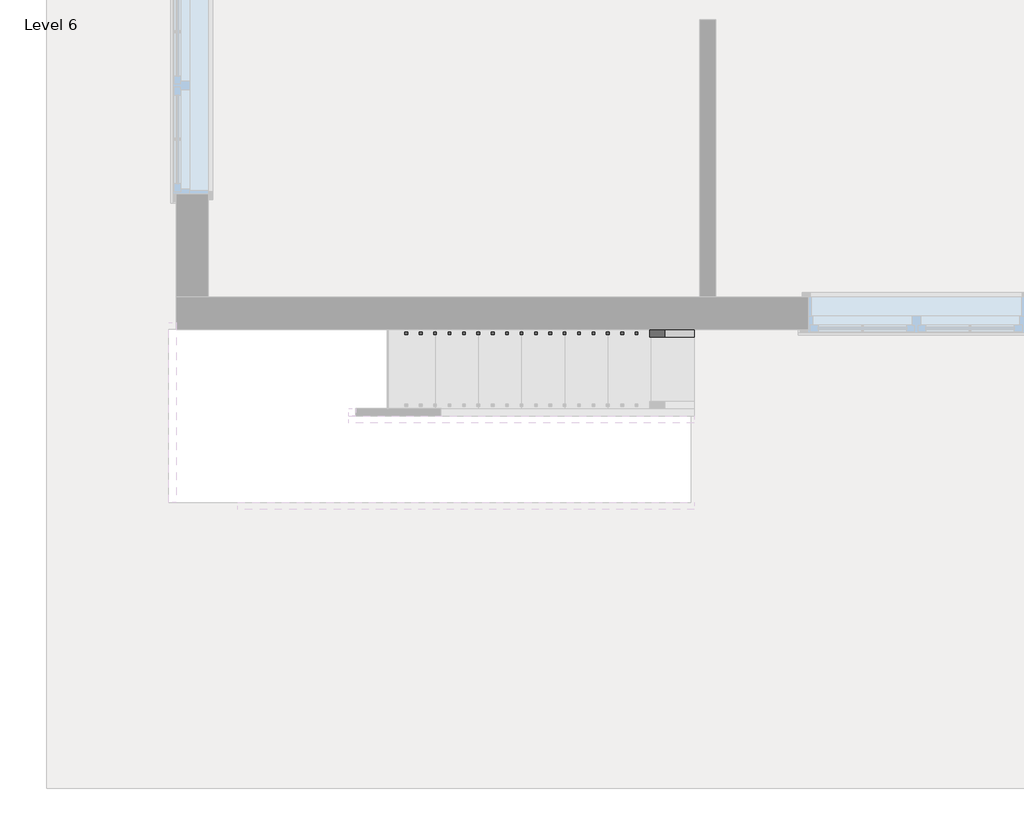
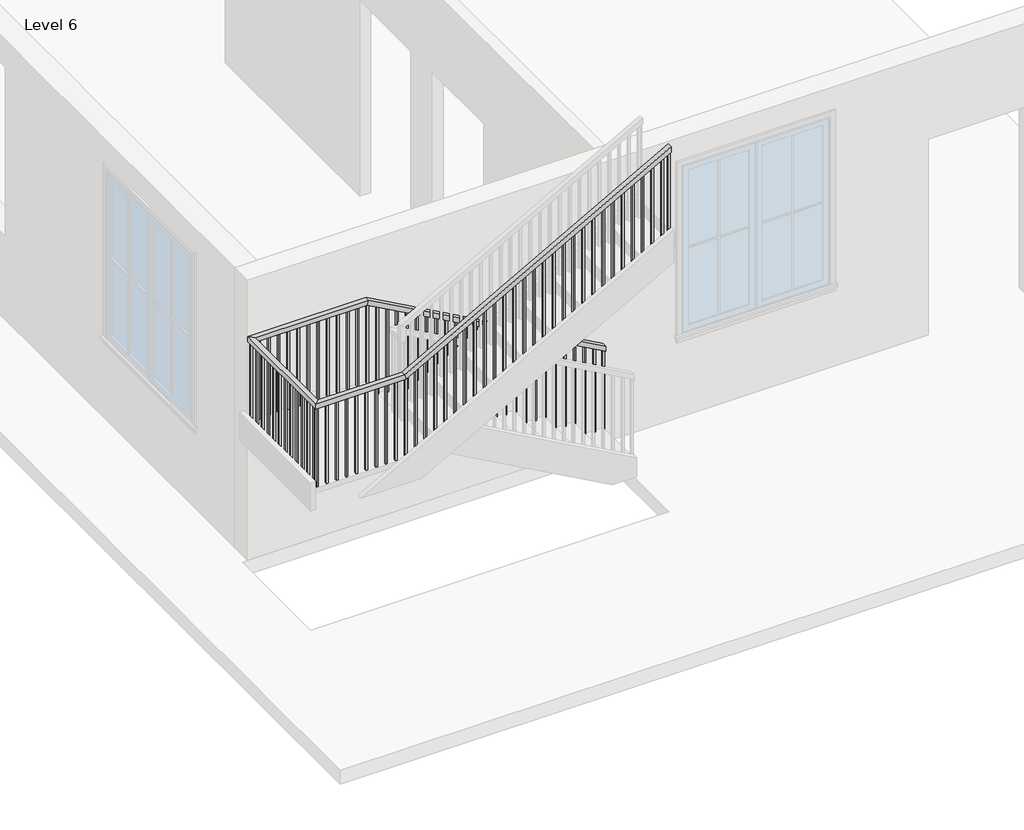
# One storey, part 2 of 3: 1 railing.
"""IFC4 building model written with IfcOpenShell, lengths in millimetres."""

from ifc_helpers import new_model, si_unit, frame, origin, place, context, project, spatial, polyline, outline, extrude, faceted_brep, element, save

model = new_model("IFC4")

# Units and contexts
model_context = context("Model", 3, world=origin())
ifc_project = project(units=[si_unit("LENGTHUNIT", "METRE", prefix="MILLI")], contexts=[model_context])

# Site, building, storey
site = spatial("IfcSite", under=ifc_project)
building = spatial("IfcBuilding", under=site)
storey = spatial("IfcBuildingStorey", under=building, Name="Level 6", Elevation=12801.6)

# Railing
placement = place(None, origin())
element("IfcRailing", 1, ObjectType="Handrail - Rectangular", at=placement, inside=storey, context=model_context, shape_type="SolidModel", body=[
    faceted_brep([(-1805.9198569, -5357.1933037, 13885.3333333), (-1805.9198569, -5357.1933037, 13827.220221), (-1805.9198569, -5306.3933037, 13827.220221), (-1805.9198569, -5306.3933037, 13885.3333333), (-4244.3198569, -5357.1933037, 15240.0), (-4257.4834592, -5357.1933037, 15189.2), (-4257.4834592, -5306.3933037, 15189.2), (-4244.3198569, -5306.3933037, 15240.0), (-5412.7198569, -5357.1933037, 15240.0), (-5412.7198569, -5357.1933037, 15189.2), (-5463.5198569, -5306.3933037, 15189.2), (-5463.5198569, -5306.3933037, 15240.0), (-5412.7198569, -6474.7933037, 15240.0), (-5412.7198569, -6474.7933037, 15189.2), (-5463.5198569, -6525.5933037, 15189.2), (-5463.5198569, -6525.5933037, 15240.0), (-4549.1198569, -6474.7933037, 15240.0), (-4535.9562547, -6474.7933037, 15189.2), (-4535.9562547, -6525.5933037, 15189.2), (-4549.1198569, -6525.5933037, 15240.0), (-1805.9198569, -6474.7933037, 16764.0), (-1805.9198569, -6525.5933037, 16764.0), (-1805.9198569, -6525.5933037, 16705.8868876), (-1805.9198569, -6474.7933037, 16705.8868876)], [[[0, 1, 2, 3]], [[1, 0, 4, 5]], [[2, 1, 5, 6]], [[3, 2, 6, 7]], [[0, 3, 7, 4]], [[5, 4, 8, 9]], [[6, 5, 9, 10]], [[7, 6, 10, 11]], [[4, 7, 11, 8]], [[9, 8, 12, 13]], [[10, 9, 13, 14]], [[11, 10, 14, 15]], [[8, 11, 15, 12]], [[13, 12, 16, 17]], [[14, 13, 17, 18]], [[15, 14, 18, 19]], [[12, 15, 19, 16]], [[20, 21, 22, 23]], [[17, 16, 20, 23]], [[18, 17, 23, 22]], [[19, 18, 22, 21]], [[16, 19, 21, 20]]]),
    extrude(outline(polyline([(16668.845221, -1872.5948569), (16658.2618876, -1891.6448569), (15680.2666667, -1891.6448569), (15680.2666667, -1872.5948569), (16668.845221, -1872.5948569)])), frame((0.0, -6509.7183037, 0.0), z_axis=(0.0, 1.0, 0.0), x_axis=(0.0, 0.0, 1.0)), (0.0, 0.0, 1.0), 19.05),
    extrude(outline(polyline([(16612.4007765, -1974.1948569), (16601.8174432, -1993.2448569), (15680.2666667, -1993.2448569), (15680.2666667, -1974.1948569), (16612.4007765, -1974.1948569)])), frame((0.0, -6509.7183037, 0.0), z_axis=(0.0, 1.0, 0.0), x_axis=(0.0, 0.0, 1.0)), (0.0, 0.0, 1.0), 19.05),
    extrude(outline(polyline([(16555.9563321, -2075.7948569), (16545.3729988, -2094.8448569), (15680.2666667, -2094.8448569), (15680.2666667, -2075.7948569), (16555.9563321, -2075.7948569)])), frame((0.0, -6509.7183037, 0.0), z_axis=(0.0, 1.0, 0.0), x_axis=(0.0, 0.0, 1.0)), (0.0, 0.0, 1.0), 19.05),
    extrude(outline(polyline([(16499.5118876, -2177.3948569), (16488.9285543, -2196.4448569), (15510.9333333, -2196.4448569), (15510.9333333, -2177.3948569), (16499.5118876, -2177.3948569)])), frame((0.0, -6509.7183037, 0.0), z_axis=(0.0, 1.0, 0.0), x_axis=(0.0, 0.0, 1.0)), (0.0, 0.0, 1.0), 19.05),
    extrude(outline(polyline([(16443.0674432, -2278.9948569), (16432.4841099, -2298.0448569), (15510.9333333, -2298.0448569), (15510.9333333, -2278.9948569), (16443.0674432, -2278.9948569)])), frame((0.0, -6509.7183037, 0.0), z_axis=(0.0, 1.0, 0.0), x_axis=(0.0, 0.0, 1.0)), (0.0, 0.0, 1.0), 19.05),
    extrude(outline(polyline([(16386.6229988, -2380.5948569), (16376.0396654, -2399.6448569), (15510.9333333, -2399.6448569), (15510.9333333, -2380.5948569), (16386.6229988, -2380.5948569)])), frame((0.0, -6509.7183037, 0.0), z_axis=(0.0, 1.0, 0.0), x_axis=(0.0, 0.0, 1.0)), (0.0, 0.0, 1.0), 19.05),
    extrude(outline(polyline([(16330.1785543, -2482.1948569), (16319.595221, -2501.2448569), (15341.6, -2501.2448569), (15341.6, -2482.1948569), (16330.1785543, -2482.1948569)])), frame((0.0, -6509.7183037, 0.0), z_axis=(0.0, 1.0, 0.0), x_axis=(0.0, 0.0, 1.0)), (0.0, 0.0, 1.0), 19.05),
    extrude(outline(polyline([(16273.7341099, -2583.7948569), (16263.1507765, -2602.8448569), (15341.6, -2602.8448569), (15341.6, -2583.7948569), (16273.7341099, -2583.7948569)])), frame((0.0, -6509.7183037, 0.0), z_axis=(0.0, 1.0, 0.0), x_axis=(0.0, 0.0, 1.0)), (0.0, 0.0, 1.0), 19.05),
    extrude(outline(polyline([(16217.2896654, -2685.3948569), (16206.7063321, -2704.4448569), (15341.6, -2704.4448569), (15341.6, -2685.3948569), (16217.2896654, -2685.3948569)])), frame((0.0, -6509.7183037, 0.0), z_axis=(0.0, 1.0, 0.0), x_axis=(0.0, 0.0, 1.0)), (0.0, 0.0, 1.0), 19.05),
    extrude(outline(polyline([(16160.845221, -2786.9948569), (16150.2618876, -2806.0448569), (15172.2666667, -2806.0448569), (15172.2666667, -2786.9948569), (16160.845221, -2786.9948569)])), frame((0.0, -6509.7183037, 0.0), z_axis=(0.0, 1.0, 0.0), x_axis=(0.0, 0.0, 1.0)), (0.0, 0.0, 1.0), 19.05),
    extrude(outline(polyline([(16104.4007765, -2888.5948569), (16093.8174432, -2907.6448569), (15172.2666667, -2907.6448569), (15172.2666667, -2888.5948569), (16104.4007765, -2888.5948569)])), frame((0.0, -6509.7183037, 0.0), z_axis=(0.0, 1.0, 0.0), x_axis=(0.0, 0.0, 1.0)), (0.0, 0.0, 1.0), 19.05),
    extrude(outline(polyline([(16047.9563321, -2990.1948569), (16037.3729988, -3009.2448569), (15172.2666667, -3009.2448569), (15172.2666667, -2990.1948569), (16047.9563321, -2990.1948569)])), frame((0.0, -6509.7183037, 0.0), z_axis=(0.0, 1.0, 0.0), x_axis=(0.0, 0.0, 1.0)), (0.0, 0.0, 1.0), 19.05),
    extrude(outline(polyline([(15991.5118876, -3091.7948569), (15980.9285543, -3110.8448569), (15002.9333333, -3110.8448569), (15002.9333333, -3091.7948569), (15991.5118876, -3091.7948569)])), frame((0.0, -6509.7183037, 0.0), z_axis=(0.0, 1.0, 0.0), x_axis=(0.0, 0.0, 1.0)), (0.0, 0.0, 1.0), 19.05),
    extrude(outline(polyline([(15935.0674432, -3193.3948569), (15924.4841099, -3212.4448569), (15002.9333333, -3212.4448569), (15002.9333333, -3193.3948569), (15935.0674432, -3193.3948569)])), frame((0.0, -6509.7183037, 0.0), z_axis=(0.0, 1.0, 0.0), x_axis=(0.0, 0.0, 1.0)), (0.0, 0.0, 1.0), 19.05),
    extrude(outline(polyline([(15878.6229988, -3294.9948569), (15868.0396654, -3314.0448569), (15002.9333333, -3314.0448569), (15002.9333333, -3294.9948569), (15878.6229988, -3294.9948569)])), frame((0.0, -6509.7183037, 0.0), z_axis=(0.0, 1.0, 0.0), x_axis=(0.0, 0.0, 1.0)), (0.0, 0.0, 1.0), 19.05),
    extrude(outline(polyline([(15822.1785543, -3396.5948569), (15811.595221, -3415.6448569), (14833.6, -3415.6448569), (14833.6, -3396.5948569), (15822.1785543, -3396.5948569)])), frame((0.0, -6509.7183037, 0.0), z_axis=(0.0, 1.0, 0.0), x_axis=(0.0, 0.0, 1.0)), (0.0, 0.0, 1.0), 19.05),
    extrude(outline(polyline([(15765.7341099, -3498.1948569), (15755.1507765, -3517.2448569), (14833.6, -3517.2448569), (14833.6, -3498.1948569), (15765.7341099, -3498.1948569)])), frame((0.0, -6509.7183037, 0.0), z_axis=(0.0, 1.0, 0.0), x_axis=(0.0, 0.0, 1.0)), (0.0, 0.0, 1.0), 19.05),
    extrude(outline(polyline([(15709.2896654, -3599.7948569), (15698.7063321, -3618.8448569), (14833.6, -3618.8448569), (14833.6, -3599.7948569), (15709.2896654, -3599.7948569)])), frame((0.0, -6509.7183037, 0.0), z_axis=(0.0, 1.0, 0.0), x_axis=(0.0, 0.0, 1.0)), (0.0, 0.0, 1.0), 19.05),
    extrude(outline(polyline([(15652.845221, -3701.3948569), (15642.2618876, -3720.4448569), (14664.2666667, -3720.4448569), (14664.2666667, -3701.3948569), (15652.845221, -3701.3948569)])), frame((0.0, -6509.7183037, 0.0), z_axis=(0.0, 1.0, 0.0), x_axis=(0.0, 0.0, 1.0)), (0.0, 0.0, 1.0), 19.05),
    extrude(outline(polyline([(15596.4007765, -3802.9948569), (15585.8174432, -3822.0448569), (14664.2666667, -3822.0448569), (14664.2666667, -3802.9948569), (15596.4007765, -3802.9948569)])), frame((0.0, -6509.7183037, 0.0), z_axis=(0.0, 1.0, 0.0), x_axis=(0.0, 0.0, 1.0)), (0.0, 0.0, 1.0), 19.05),
    extrude(outline(polyline([(15539.9563321, -3904.5948569), (15529.3729988, -3923.6448569), (14664.2666667, -3923.6448569), (14664.2666667, -3904.5948569), (15539.9563321, -3904.5948569)])), frame((0.0, -6509.7183037, 0.0), z_axis=(0.0, 1.0, 0.0), x_axis=(0.0, 0.0, 1.0)), (0.0, 0.0, 1.0), 19.05),
    extrude(outline(polyline([(15483.5118876, -4006.1948569), (15472.9285543, -4025.2448569), (14494.9333333, -4025.2448569), (14494.9333333, -4006.1948569), (15483.5118876, -4006.1948569)])), frame((0.0, -6509.7183037, 0.0), z_axis=(0.0, 1.0, 0.0), x_axis=(0.0, 0.0, 1.0)), (0.0, 0.0, 1.0), 19.05),
    extrude(outline(polyline([(15427.0674432, -4107.7948569), (15416.4841099, -4126.8448569), (14494.9333333, -4126.8448569), (14494.9333333, -4107.7948569), (15427.0674432, -4107.7948569)])), frame((0.0, -6509.7183037, 0.0), z_axis=(0.0, 1.0, 0.0), x_axis=(0.0, 0.0, 1.0)), (0.0, 0.0, 1.0), 19.05),
    extrude(outline(polyline([(15370.6229988, -4209.3948569), (15360.0396654, -4228.4448569), (14494.9333333, -4228.4448569), (14494.9333333, -4209.3948569), (15370.6229988, -4209.3948569)])), frame((0.0, -6509.7183037, 0.0), z_axis=(0.0, 1.0, 0.0), x_axis=(0.0, 0.0, 1.0)), (0.0, 0.0, 1.0), 19.05),
    extrude(outline(polyline([(15314.1785543, -4310.9948569), (15303.595221, -4330.0448569), (14325.6, -4330.0448569), (14325.6, -4310.9948569), (15314.1785543, -4310.9948569)])), frame((0.0, -6509.7183037, 0.0), z_axis=(0.0, 1.0, 0.0), x_axis=(0.0, 0.0, 1.0)), (0.0, 0.0, 1.0), 19.05),
    extrude(outline(polyline([(15257.7341099, -4412.5948569), (15247.1507765, -4431.6448569), (14325.6, -4431.6448569), (14325.6, -4412.5948569), (15257.7341099, -4412.5948569)])), frame((0.0, -6509.7183037, 0.0), z_axis=(0.0, 1.0, 0.0), x_axis=(0.0, 0.0, 1.0)), (0.0, 0.0, 1.0), 19.05),
    extrude(outline(polyline([(15201.2896654, -4514.1948569), (15190.7063321, -4533.2448569), (14325.6, -4533.2448569), (14325.6, -4514.1948569), (15201.2896654, -4514.1948569)])), frame((0.0, -6509.7183037, 0.0), z_axis=(0.0, 1.0, 0.0), x_axis=(0.0, 0.0, 1.0)), (0.0, 0.0, 1.0), 19.05),
    extrude(outline(polyline([(-4634.8448569, -6509.7183037), (-4634.8448569, -6490.6683037), (-4615.7948569, -6490.6683037), (-4615.7948569, -6509.7183037), (-4634.8448569, -6509.7183037)])), frame((0.0, 0.0, 14325.6), z_axis=(0.0, 0.0, 1.0), x_axis=(1.0, 0.0, 0.0)), (0.0, 0.0, 1.0), 863.6),
    extrude(outline(polyline([(-4736.4448569, -6509.7183037), (-4736.4448569, -6490.6683037), (-4717.3948569, -6490.6683037), (-4717.3948569, -6509.7183037), (-4736.4448569, -6509.7183037)])), frame((0.0, 0.0, 14325.6), z_axis=(0.0, 0.0, 1.0), x_axis=(1.0, 0.0, 0.0)), (0.0, 0.0, 1.0), 863.6),
    extrude(outline(polyline([(-4838.0448569, -6509.7183037), (-4838.0448569, -6490.6683037), (-4818.9948569, -6490.6683037), (-4818.9948569, -6509.7183037), (-4838.0448569, -6509.7183037)])), frame((0.0, 0.0, 14325.6), z_axis=(0.0, 0.0, 1.0), x_axis=(1.0, 0.0, 0.0)), (0.0, 0.0, 1.0), 863.6),
    extrude(outline(polyline([(-4939.6448569, -6509.7183037), (-4939.6448569, -6490.6683037), (-4920.5948569, -6490.6683037), (-4920.5948569, -6509.7183037), (-4939.6448569, -6509.7183037)])), frame((0.0, 0.0, 14325.6), z_axis=(0.0, 0.0, 1.0), x_axis=(1.0, 0.0, 0.0)), (0.0, 0.0, 1.0), 863.6),
    extrude(outline(polyline([(-5041.2448569, -6509.7183037), (-5041.2448569, -6490.6683037), (-5022.1948569, -6490.6683037), (-5022.1948569, -6509.7183037), (-5041.2448569, -6509.7183037)])), frame((0.0, 0.0, 14325.6), z_axis=(0.0, 0.0, 1.0), x_axis=(1.0, 0.0, 0.0)), (0.0, 0.0, 1.0), 863.6),
    extrude(outline(polyline([(-5142.8448569, -6509.7183037), (-5142.8448569, -6490.6683037), (-5123.7948569, -6490.6683037), (-5123.7948569, -6509.7183037), (-5142.8448569, -6509.7183037)])), frame((0.0, 0.0, 14325.6), z_axis=(0.0, 0.0, 1.0), x_axis=(1.0, 0.0, 0.0)), (0.0, 0.0, 1.0), 863.6),
    extrude(outline(polyline([(-5244.4448569, -6509.7183037), (-5244.4448569, -6490.6683037), (-5225.3948569, -6490.6683037), (-5225.3948569, -6509.7183037), (-5244.4448569, -6509.7183037)])), frame((0.0, 0.0, 14325.6), z_axis=(0.0, 0.0, 1.0), x_axis=(1.0, 0.0, 0.0)), (0.0, 0.0, 1.0), 863.6),
    extrude(outline(polyline([(-5346.0448569, -6509.7183037), (-5346.0448569, -6490.6683037), (-5326.9948569, -6490.6683037), (-5326.9948569, -6509.7183037), (-5346.0448569, -6509.7183037)])), frame((0.0, 0.0, 14325.6), z_axis=(0.0, 0.0, 1.0), x_axis=(1.0, 0.0, 0.0)), (0.0, 0.0, 1.0), 863.6),
    extrude(outline(polyline([(-5447.6448569, -6439.8683037), (-5428.5948569, -6439.8683037), (-5428.5948569, -6458.9183037), (-5447.6448569, -6458.9183037), (-5447.6448569, -6439.8683037)])), frame((0.0, 0.0, 14325.6), z_axis=(0.0, 0.0, 1.0), x_axis=(1.0, 0.0, 0.0)), (0.0, 0.0, 1.0), 863.6),
    extrude(outline(polyline([(-5447.6448569, -6338.2683037), (-5428.5948569, -6338.2683037), (-5428.5948569, -6357.3183037), (-5447.6448569, -6357.3183037), (-5447.6448569, -6338.2683037)])), frame((0.0, 0.0, 14325.6), z_axis=(0.0, 0.0, 1.0), x_axis=(1.0, 0.0, 0.0)), (0.0, 0.0, 1.0), 863.6),
    extrude(outline(polyline([(-5447.6448569, -6236.6683037), (-5428.5948569, -6236.6683037), (-5428.5948569, -6255.7183037), (-5447.6448569, -6255.7183037), (-5447.6448569, -6236.6683037)])), frame((0.0, 0.0, 14325.6), z_axis=(0.0, 0.0, 1.0), x_axis=(1.0, 0.0, 0.0)), (0.0, 0.0, 1.0), 863.6),
    extrude(outline(polyline([(-5447.6448569, -6135.0683037), (-5428.5948569, -6135.0683037), (-5428.5948569, -6154.1183037), (-5447.6448569, -6154.1183037), (-5447.6448569, -6135.0683037)])), frame((0.0, 0.0, 14325.6), z_axis=(0.0, 0.0, 1.0), x_axis=(1.0, 0.0, 0.0)), (0.0, 0.0, 1.0), 863.6),
    extrude(outline(polyline([(-5447.6448569, -6033.4683037), (-5428.5948569, -6033.4683037), (-5428.5948569, -6052.5183037), (-5447.6448569, -6052.5183037), (-5447.6448569, -6033.4683037)])), frame((0.0, 0.0, 14325.6), z_axis=(0.0, 0.0, 1.0), x_axis=(1.0, 0.0, 0.0)), (0.0, 0.0, 1.0), 863.6),
    extrude(outline(polyline([(-5447.6448569, -5931.8683037), (-5428.5948569, -5931.8683037), (-5428.5948569, -5950.9183037), (-5447.6448569, -5950.9183037), (-5447.6448569, -5931.8683037)])), frame((0.0, 0.0, 14325.6), z_axis=(0.0, 0.0, 1.0), x_axis=(1.0, 0.0, 0.0)), (0.0, 0.0, 1.0), 863.6),
    extrude(outline(polyline([(-5447.6448569, -5830.2683037), (-5428.5948569, -5830.2683037), (-5428.5948569, -5849.3183037), (-5447.6448569, -5849.3183037), (-5447.6448569, -5830.2683037)])), frame((0.0, 0.0, 14325.6), z_axis=(0.0, 0.0, 1.0), x_axis=(1.0, 0.0, 0.0)), (0.0, 0.0, 1.0), 863.6),
    extrude(outline(polyline([(-5447.6448569, -5728.6683037), (-5428.5948569, -5728.6683037), (-5428.5948569, -5747.7183037), (-5447.6448569, -5747.7183037), (-5447.6448569, -5728.6683037)])), frame((0.0, 0.0, 14325.6), z_axis=(0.0, 0.0, 1.0), x_axis=(1.0, 0.0, 0.0)), (0.0, 0.0, 1.0), 863.6),
    extrude(outline(polyline([(-5447.6448569, -5627.0683037), (-5428.5948569, -5627.0683037), (-5428.5948569, -5646.1183037), (-5447.6448569, -5646.1183037), (-5447.6448569, -5627.0683037)])), frame((0.0, 0.0, 14325.6), z_axis=(0.0, 0.0, 1.0), x_axis=(1.0, 0.0, 0.0)), (0.0, 0.0, 1.0), 863.6),
    extrude(outline(polyline([(-5447.6448569, -5525.4683037), (-5428.5948569, -5525.4683037), (-5428.5948569, -5544.5183037), (-5447.6448569, -5544.5183037), (-5447.6448569, -5525.4683037)])), frame((0.0, 0.0, 14325.6), z_axis=(0.0, 0.0, 1.0), x_axis=(1.0, 0.0, 0.0)), (0.0, 0.0, 1.0), 863.6),
    extrude(outline(polyline([(-5447.6448569, -5423.8683037), (-5428.5948569, -5423.8683037), (-5428.5948569, -5442.9183037), (-5447.6448569, -5442.9183037), (-5447.6448569, -5423.8683037)])), frame((0.0, 0.0, 14325.6), z_axis=(0.0, 0.0, 1.0), x_axis=(1.0, 0.0, 0.0)), (0.0, 0.0, 1.0), 863.6),
    extrude(outline(polyline([(-5352.3948569, -5322.2683037), (-5352.3948569, -5341.3183037), (-5371.4448569, -5341.3183037), (-5371.4448569, -5322.2683037), (-5352.3948569, -5322.2683037)])), frame((0.0, 0.0, 14325.6), z_axis=(0.0, 0.0, 1.0), x_axis=(1.0, 0.0, 0.0)), (0.0, 0.0, 1.0), 863.6),
    extrude(outline(polyline([(-5250.7948569, -5322.2683037), (-5250.7948569, -5341.3183037), (-5269.8448569, -5341.3183037), (-5269.8448569, -5322.2683037), (-5250.7948569, -5322.2683037)])), frame((0.0, 0.0, 14325.6), z_axis=(0.0, 0.0, 1.0), x_axis=(1.0, 0.0, 0.0)), (0.0, 0.0, 1.0), 863.6),
    extrude(outline(polyline([(-5149.1948569, -5322.2683037), (-5149.1948569, -5341.3183037), (-5168.2448569, -5341.3183037), (-5168.2448569, -5322.2683037), (-5149.1948569, -5322.2683037)])), frame((0.0, 0.0, 14325.6), z_axis=(0.0, 0.0, 1.0), x_axis=(1.0, 0.0, 0.0)), (0.0, 0.0, 1.0), 863.6),
    extrude(outline(polyline([(-5047.5948569, -5322.2683037), (-5047.5948569, -5341.3183037), (-5066.6448569, -5341.3183037), (-5066.6448569, -5322.2683037), (-5047.5948569, -5322.2683037)])), frame((0.0, 0.0, 14325.6), z_axis=(0.0, 0.0, 1.0), x_axis=(1.0, 0.0, 0.0)), (0.0, 0.0, 1.0), 863.6),
    extrude(outline(polyline([(-4945.9948569, -5322.2683037), (-4945.9948569, -5341.3183037), (-4965.0448569, -5341.3183037), (-4965.0448569, -5322.2683037), (-4945.9948569, -5322.2683037)])), frame((0.0, 0.0, 14325.6), z_axis=(0.0, 0.0, 1.0), x_axis=(1.0, 0.0, 0.0)), (0.0, 0.0, 1.0), 863.6),
    extrude(outline(polyline([(-4844.3948569, -5322.2683037), (-4844.3948569, -5341.3183037), (-4863.4448569, -5341.3183037), (-4863.4448569, -5322.2683037), (-4844.3948569, -5322.2683037)])), frame((0.0, 0.0, 14325.6), z_axis=(0.0, 0.0, 1.0), x_axis=(1.0, 0.0, 0.0)), (0.0, 0.0, 1.0), 863.6),
    extrude(outline(polyline([(-4742.7948569, -5322.2683037), (-4742.7948569, -5341.3183037), (-4761.8448569, -5341.3183037), (-4761.8448569, -5322.2683037), (-4742.7948569, -5322.2683037)])), frame((0.0, 0.0, 14325.6), z_axis=(0.0, 0.0, 1.0), x_axis=(1.0, 0.0, 0.0)), (0.0, 0.0, 1.0), 863.6),
    extrude(outline(polyline([(-4641.1948569, -5322.2683037), (-4641.1948569, -5341.3183037), (-4660.2448569, -5341.3183037), (-4660.2448569, -5322.2683037), (-4641.1948569, -5322.2683037)])), frame((0.0, 0.0, 14325.6), z_axis=(0.0, 0.0, 1.0), x_axis=(1.0, 0.0, 0.0)), (0.0, 0.0, 1.0), 863.6),
    extrude(outline(polyline([(-4539.5948569, -5322.2683037), (-4539.5948569, -5341.3183037), (-4558.6448569, -5341.3183037), (-4558.6448569, -5322.2683037), (-4539.5948569, -5322.2683037)])), frame((0.0, 0.0, 14325.6), z_axis=(0.0, 0.0, 1.0), x_axis=(1.0, 0.0, 0.0)), (0.0, 0.0, 1.0), 863.6),
    extrude(outline(polyline([(-4437.9948569, -5322.2683037), (-4437.9948569, -5341.3183037), (-4457.0448569, -5341.3183037), (-4457.0448569, -5322.2683037), (-4437.9948569, -5322.2683037)])), frame((0.0, 0.0, 14325.6), z_axis=(0.0, 0.0, 1.0), x_axis=(1.0, 0.0, 0.0)), (0.0, 0.0, 1.0), 863.6),
    extrude(outline(polyline([(-4336.3948569, -5322.2683037), (-4336.3948569, -5341.3183037), (-4355.4448569, -5341.3183037), (-4355.4448569, -5322.2683037), (-4336.3948569, -5322.2683037)])), frame((0.0, 0.0, 14325.6), z_axis=(0.0, 0.0, 1.0), x_axis=(1.0, 0.0, 0.0)), (0.0, 0.0, 1.0), 863.6),
    extrude(outline(polyline([(15176.595221, -4234.7948569), (15187.1785543, -4253.8448569), (14325.6, -4253.8448569), (14325.6, -4234.7948569), (15176.595221, -4234.7948569)])), frame((0.0, -5341.3183037, 0.0), z_axis=(0.0, 1.0, 0.0), x_axis=(0.0, 0.0, 1.0)), (0.0, 0.0, 1.0), 19.05),
    extrude(outline(polyline([(15120.1507765, -4133.1948569), (15130.7341099, -4152.2448569), (14156.2666667, -4152.2448569), (14156.2666667, -4133.1948569), (15120.1507765, -4133.1948569)])), frame((0.0, -5341.3183037, 0.0), z_axis=(0.0, 1.0, 0.0), x_axis=(0.0, 0.0, 1.0)), (0.0, 0.0, 1.0), 19.05),
    extrude(outline(polyline([(15063.7063321, -4031.5948569), (15074.2896654, -4050.6448569), (14156.2666667, -4050.6448569), (14156.2666667, -4031.5948569), (15063.7063321, -4031.5948569)])), frame((0.0, -5341.3183037, 0.0), z_axis=(0.0, 1.0, 0.0), x_axis=(0.0, 0.0, 1.0)), (0.0, 0.0, 1.0), 19.05),
    extrude(outline(polyline([(15007.2618876, -3929.9948569), (15017.845221, -3949.0448569), (14156.2666667, -3949.0448569), (14156.2666667, -3929.9948569), (15007.2618876, -3929.9948569)])), frame((0.0, -5341.3183037, 0.0), z_axis=(0.0, 1.0, 0.0), x_axis=(0.0, 0.0, 1.0)), (0.0, 0.0, 1.0), 19.05),
    extrude(outline(polyline([(14950.8174432, -3828.3948569), (14961.4007765, -3847.4448569), (13986.9333333, -3847.4448569), (13986.9333333, -3828.3948569), (14950.8174432, -3828.3948569)])), frame((0.0, -5341.3183037, 0.0), z_axis=(0.0, 1.0, 0.0), x_axis=(0.0, 0.0, 1.0)), (0.0, 0.0, 1.0), 19.05),
    extrude(outline(polyline([(14894.3729988, -3726.7948569), (14904.9563321, -3745.8448569), (13986.9333333, -3745.8448569), (13986.9333333, -3726.7948569), (14894.3729988, -3726.7948569)])), frame((0.0, -5341.3183037, 0.0), z_axis=(0.0, 1.0, 0.0), x_axis=(0.0, 0.0, 1.0)), (0.0, 0.0, 1.0), 19.05),
    extrude(outline(polyline([(14837.9285543, -3625.1948569), (14848.5118876, -3644.2448569), (13986.9333333, -3644.2448569), (13986.9333333, -3625.1948569), (14837.9285543, -3625.1948569)])), frame((0.0, -5341.3183037, 0.0), z_axis=(0.0, 1.0, 0.0), x_axis=(0.0, 0.0, 1.0)), (0.0, 0.0, 1.0), 19.05),
    extrude(outline(polyline([(14781.4841099, -3523.5948569), (14792.0674432, -3542.6448569), (13817.6, -3542.6448569), (13817.6, -3523.5948569), (14781.4841099, -3523.5948569)])), frame((0.0, -5341.3183037, 0.0), z_axis=(0.0, 1.0, 0.0), x_axis=(0.0, 0.0, 1.0)), (0.0, 0.0, 1.0), 19.05),
    extrude(outline(polyline([(14725.0396654, -3421.9948569), (14735.6229988, -3441.0448569), (13817.6, -3441.0448569), (13817.6, -3421.9948569), (14725.0396654, -3421.9948569)])), frame((0.0, -5341.3183037, 0.0), z_axis=(0.0, 1.0, 0.0), x_axis=(0.0, 0.0, 1.0)), (0.0, 0.0, 1.0), 19.05),
    extrude(outline(polyline([(14668.595221, -3320.3948569), (14679.1785543, -3339.4448569), (13817.6, -3339.4448569), (13817.6, -3320.3948569), (14668.595221, -3320.3948569)])), frame((0.0, -5341.3183037, 0.0), z_axis=(0.0, 1.0, 0.0), x_axis=(0.0, 0.0, 1.0)), (0.0, 0.0, 1.0), 19.05),
    extrude(outline(polyline([(14612.1507765, -3218.7948569), (14622.7341099, -3237.8448569), (13648.2666667, -3237.8448569), (13648.2666667, -3218.7948569), (14612.1507765, -3218.7948569)])), frame((0.0, -5341.3183037, 0.0), z_axis=(0.0, 1.0, 0.0), x_axis=(0.0, 0.0, 1.0)), (0.0, 0.0, 1.0), 19.05),
    extrude(outline(polyline([(14555.7063321, -3117.1948569), (14566.2896654, -3136.2448569), (13648.2666667, -3136.2448569), (13648.2666667, -3117.1948569), (14555.7063321, -3117.1948569)])), frame((0.0, -5341.3183037, 0.0), z_axis=(0.0, 1.0, 0.0), x_axis=(0.0, 0.0, 1.0)), (0.0, 0.0, 1.0), 19.05),
    extrude(outline(polyline([(14499.2618876, -3015.5948569), (14509.845221, -3034.6448569), (13648.2666667, -3034.6448569), (13648.2666667, -3015.5948569), (14499.2618876, -3015.5948569)])), frame((0.0, -5341.3183037, 0.0), z_axis=(0.0, 1.0, 0.0), x_axis=(0.0, 0.0, 1.0)), (0.0, 0.0, 1.0), 19.05),
    extrude(outline(polyline([(14442.8174432, -2913.9948569), (14453.4007765, -2933.0448569), (13478.9333333, -2933.0448569), (13478.9333333, -2913.9948569), (14442.8174432, -2913.9948569)])), frame((0.0, -5341.3183037, 0.0), z_axis=(0.0, 1.0, 0.0), x_axis=(0.0, 0.0, 1.0)), (0.0, 0.0, 1.0), 19.05),
    extrude(outline(polyline([(14386.3729988, -2812.3948569), (14396.9563321, -2831.4448569), (13478.9333333, -2831.4448569), (13478.9333333, -2812.3948569), (14386.3729988, -2812.3948569)])), frame((0.0, -5341.3183037, 0.0), z_axis=(0.0, 1.0, 0.0), x_axis=(0.0, 0.0, 1.0)), (0.0, 0.0, 1.0), 19.05),
    extrude(outline(polyline([(14329.9285543, -2710.7948569), (14340.5118876, -2729.8448569), (13478.9333333, -2729.8448569), (13478.9333333, -2710.7948569), (14329.9285543, -2710.7948569)])), frame((0.0, -5341.3183037, 0.0), z_axis=(0.0, 1.0, 0.0), x_axis=(0.0, 0.0, 1.0)), (0.0, 0.0, 1.0), 19.05),
    extrude(outline(polyline([(14273.4841099, -2609.1948569), (14284.0674432, -2628.2448569), (13309.6, -2628.2448569), (13309.6, -2609.1948569), (14273.4841099, -2609.1948569)])), frame((0.0, -5341.3183037, 0.0), z_axis=(0.0, 1.0, 0.0), x_axis=(0.0, 0.0, 1.0)), (0.0, 0.0, 1.0), 19.05),
    extrude(outline(polyline([(14217.0396654, -2507.5948569), (14227.6229988, -2526.6448569), (13309.6, -2526.6448569), (13309.6, -2507.5948569), (14217.0396654, -2507.5948569)])), frame((0.0, -5341.3183037, 0.0), z_axis=(0.0, 1.0, 0.0), x_axis=(0.0, 0.0, 1.0)), (0.0, 0.0, 1.0), 19.05),
    extrude(outline(polyline([(14160.595221, -2405.9948569), (14171.1785543, -2425.0448569), (13309.6, -2425.0448569), (13309.6, -2405.9948569), (14160.595221, -2405.9948569)])), frame((0.0, -5341.3183037, 0.0), z_axis=(0.0, 1.0, 0.0), x_axis=(0.0, 0.0, 1.0)), (0.0, 0.0, 1.0), 19.05),
    extrude(outline(polyline([(14104.1507765, -2304.3948569), (14114.7341099, -2323.4448569), (13140.2666667, -2323.4448569), (13140.2666667, -2304.3948569), (14104.1507765, -2304.3948569)])), frame((0.0, -5341.3183037, 0.0), z_axis=(0.0, 1.0, 0.0), x_axis=(0.0, 0.0, 1.0)), (0.0, 0.0, 1.0), 19.05),
    extrude(outline(polyline([(14047.7063321, -2202.7948569), (14058.2896654, -2221.8448569), (13140.2666667, -2221.8448569), (13140.2666667, -2202.7948569), (14047.7063321, -2202.7948569)])), frame((0.0, -5341.3183037, 0.0), z_axis=(0.0, 1.0, 0.0), x_axis=(0.0, 0.0, 1.0)), (0.0, 0.0, 1.0), 19.05),
    extrude(outline(polyline([(13991.2618876, -2101.1948569), (14001.845221, -2120.2448569), (13140.2666667, -2120.2448569), (13140.2666667, -2101.1948569), (13991.2618876, -2101.1948569)])), frame((0.0, -5341.3183037, 0.0), z_axis=(0.0, 1.0, 0.0), x_axis=(0.0, 0.0, 1.0)), (0.0, 0.0, 1.0), 19.05),
    extrude(outline(polyline([(13934.8174432, -1999.5948569), (13945.4007765, -2018.6448569), (12970.9333333, -2018.6448569), (12970.9333333, -1999.5948569), (13934.8174432, -1999.5948569)])), frame((0.0, -5341.3183037, 0.0), z_axis=(0.0, 1.0, 0.0), x_axis=(0.0, 0.0, 1.0)), (0.0, 0.0, 1.0), 19.05),
    extrude(outline(polyline([(13878.3729988, -1897.9948569), (13888.9563321, -1917.0448569), (12970.9333333, -1917.0448569), (12970.9333333, -1897.9948569), (13878.3729988, -1897.9948569)])), frame((0.0, -5341.3183037, 0.0), z_axis=(0.0, 1.0, 0.0), x_axis=(0.0, 0.0, 1.0)), (0.0, 0.0, 1.0), 19.05),
    extrude(outline(polyline([(-5447.6448569, -6490.6683037), (-5428.5948569, -6490.6683037), (-5428.5948569, -6509.7183037), (-5447.6448569, -6509.7183037), (-5447.6448569, -6490.6683037)])), frame((0.0, 0.0, 14325.6), z_axis=(0.0, 0.0, 1.0), x_axis=(1.0, 0.0, 0.0)), (0.0, 0.0, 1.0), 863.6),
    extrude(outline(polyline([(-5428.5948569, -5322.2683037), (-5428.5948569, -5341.3183037), (-5447.6448569, -5341.3183037), (-5447.6448569, -5322.2683037), (-5428.5948569, -5322.2683037)])), frame((0.0, 0.0, 14325.6), z_axis=(0.0, 0.0, 1.0), x_axis=(1.0, 0.0, 0.0)), (0.0, 0.0, 1.0), 863.6),
    extrude(outline(polyline([(16705.8868876, -1805.9198569), (16695.3035543, -1824.9698569), (15680.2666667, -1824.9698569), (15680.2666667, -1805.9198569), (16705.8868876, -1805.9198569)])), frame((0.0, -6509.7183037, 0.0), z_axis=(0.0, 1.0, 0.0), x_axis=(0.0, 0.0, 1.0)), (0.0, 0.0, 1.0), 19.05),
    extrude(outline(polyline([(13827.220221, -1805.9198569), (13837.8035543, -1824.9698569), (12970.9333333, -1824.9698569), (12970.9333333, -1805.9198569), (13827.220221, -1805.9198569)])), frame((0.0, -5341.3183037, 0.0), z_axis=(0.0, 1.0, 0.0), x_axis=(0.0, 0.0, 1.0)), (0.0, 0.0, 1.0), 19.05),
])

save(model, "model.ifc")

# Revit data of these elements
# Type "Handrail - Rectangular"
#   Assembly Code = "C2010400"
#   built-in parameter 1008612 = 0.0416667 (stored number, unit not read)
#   built-in parameter 1008611 = 0.0416667 (stored number, unit not read)
#   built-in parameter 1008609 = 0.333333 (stored number, unit not read)
#   built-in parameter 1008604 = 0.166667 (stored number, unit not read)
#   built-in parameter 1008603 = 0.166667 (stored number, unit not read)
#   Railing Height = 3' - 0"
#   built-in parameter 1008630 = 2
#   built-in parameter 1008610 = 2
#   built-in parameter 1008618 = Baluster - Square : 3/4"
# Element 1 (IfcRailing, "Handrail - Rectangular")
#   Phase Created = New Construction
